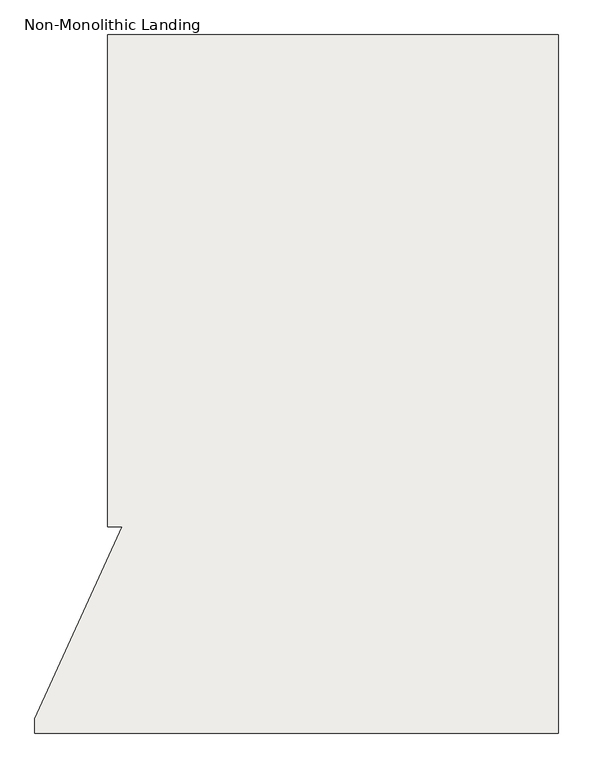
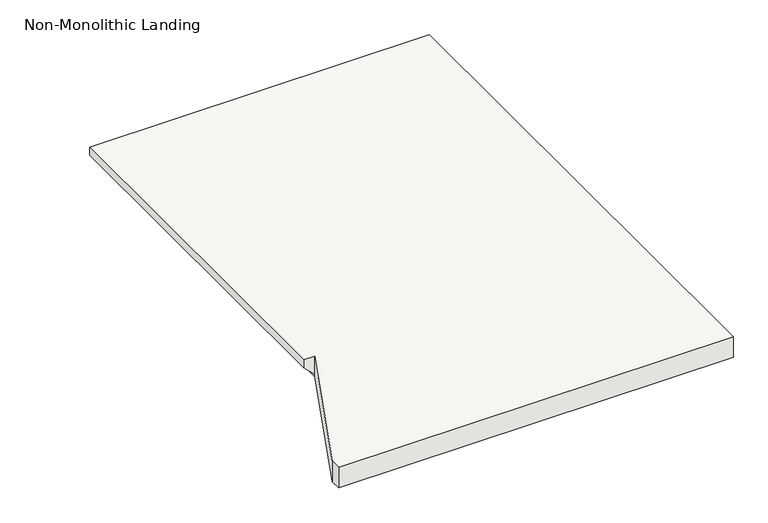
"""IFC4 building model written with IfcOpenShell, lengths in millimetres: slab geometry, Non-Monolithic Landing."""

from ifc_helpers import new_model, si_unit, origin, place, context, project, spatial, faceted_brep, source, transform, mapped, element, save


def non_monolithic_landing_39c3fcf1(model_context):
    return source(origin(), model_context, "Body", "Brep", [
        faceted_brep([(-7555.5118598, 4396.0168529, 1185.3333333), (-7555.5118598, 4396.0168529, 1166.2833333), (-7530.1118598, 4396.0168529, 1140.8833333), (-7530.1118598, 4396.0168529, 1185.3333333), (-7555.5118598, 5254.5368529, 1185.3333333), (-7555.5118598, 5254.5368529, 1166.2833333), (-7530.1118598, 5254.5368529, 1140.8833333), (-7682.5118598, 4060.7368529, 1185.3333333), (-7682.5118598, 4035.3368529, 1185.3333333), (-6768.1118598, 4035.3368529, 1185.3333333), (-6768.1118598, 4060.7368529, 1185.3333333), (-6768.1118598, 5254.5368529, 1185.3333333), (-7530.1118598, 4396.0168529, 1134.5333333), (-7530.1118598, 5254.5368529, 1134.5333333), (-6768.1118598, 5254.5368529, 1134.5333333), (-6768.1118598, 4060.7368529, 1134.5333333), (-6768.1118598, 4035.3368529, 1134.5333333), (-7682.5118598, 4035.3368529, 1134.5333333), (-7682.5118598, 4060.7368529, 1134.5333333)], [[[0, 1, 2, 3]], [[1, 0, 4, 5]], [[2, 1, 5, 6]], [[3, 7, 8, 9, 10, 11, 4, 0]], [[12, 13, 14, 15, 16, 17, 18]], [[13, 12, 2, 6]], [[7, 3, 2, 12, 18]], [[8, 7, 18, 17]], [[9, 8, 17, 16]], [[10, 9, 16, 15]], [[11, 10, 15, 14]], [[4, 11, 14, 13, 6, 5]]]),
    ])


if __name__ == "__main__":
    model = new_model("IFC4")
    model_context = context("Model", 3, world=origin())
    ifc_project = project(units=[si_unit("LENGTHUNIT", "METRE", prefix="MILLI")], contexts=[model_context])
    site = spatial("IfcSite", under=ifc_project)
    building = spatial("IfcBuilding", under=site)
    placement = place(None, origin())
    non_monolithic_landing_shape = non_monolithic_landing_39c3fcf1(model_context)
    element("IfcSlab", 1, ObjectType="Non-Monolithic Landing", at=placement, inside=building, context=model_context, shape_type="MappedRepresentation", body=[
        mapped(non_monolithic_landing_shape, transform((0.0, 0.0, 0.0), x_axis=(1.0, 0.0, 0.0), y_axis=(0.0, 1.0, 0.0), z_axis=(0.0, 0.0, 1.0))),
    ])
    save(model, "model.ifc")
